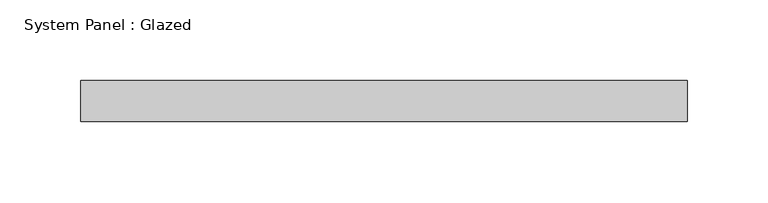
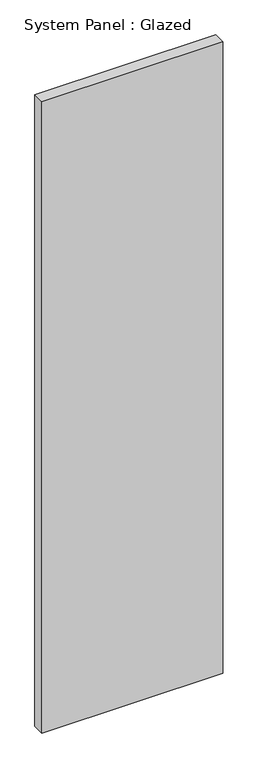
"""IFC4 building model written with IfcOpenShell, lengths in millimetres: plate geometry, System Panel : Glazed."""

from ifc_helpers import new_model, si_unit, origin, origin_with_axes, place, context, project, spatial, polyline, outline, extrude, source, transform, mapped, element, save


def system_panel_glazed_accf4d1c(model_context):
    return source(origin(), model_context, "Body", "SweptSolid", [
        extrude(outline(polyline([(187.325, 19.05), (-187.325, 19.05), (-187.325, 44.45), (187.325, 44.45), (187.325, 19.05)])), origin_with_axes(), (0.0, 0.0, 1.0), 1383.5980535),
    ])


if __name__ == "__main__":
    model = new_model("IFC4")
    model_context = context("Model", 3, world=origin())
    ifc_project = project(units=[si_unit("LENGTHUNIT", "METRE", prefix="MILLI")], contexts=[model_context])
    site = spatial("IfcSite", under=ifc_project)
    building = spatial("IfcBuilding", under=site)
    placement = place(None, origin())
    system_panel_glazed_shape = system_panel_glazed_accf4d1c(model_context)
    element("IfcPlate", 1, ObjectType="System Panel : Glazed", at=placement, inside=building, context=model_context, shape_type="MappedRepresentation", body=[
        mapped(system_panel_glazed_shape, transform((0.0, 0.0, 0.0), x_axis=(1.0, 0.0, 0.0), y_axis=(0.0, 1.0, 0.0), z_axis=(0.0, 0.0, 1.0))),
    ])
    save(model, "model.ifc")

# Revit data of these elements
# Type "System Panel : Glazed"
#   Construction Type Id = "GSP4R"
#   Analytic Construction = "1/8 in Pilkington single glazing"
#   Visual Light Transmittance = 0.9
#   Solar Heat Gain Coefficient = 0.86
#   Heat Transfer Coefficient (U) = 1.18115 BTU/(h·ft²·°F)
#   Define Thermal Properties by = 1
# Element 1 (IfcPlate, "System Panel : Glazed")
#   Materials on its faces: "Glass"
# Materials
#   "Glass": class "Glass", colour RGB 0 128 192, transparency 0.75, Description = "Soda Lime Glass", Cost = 0
